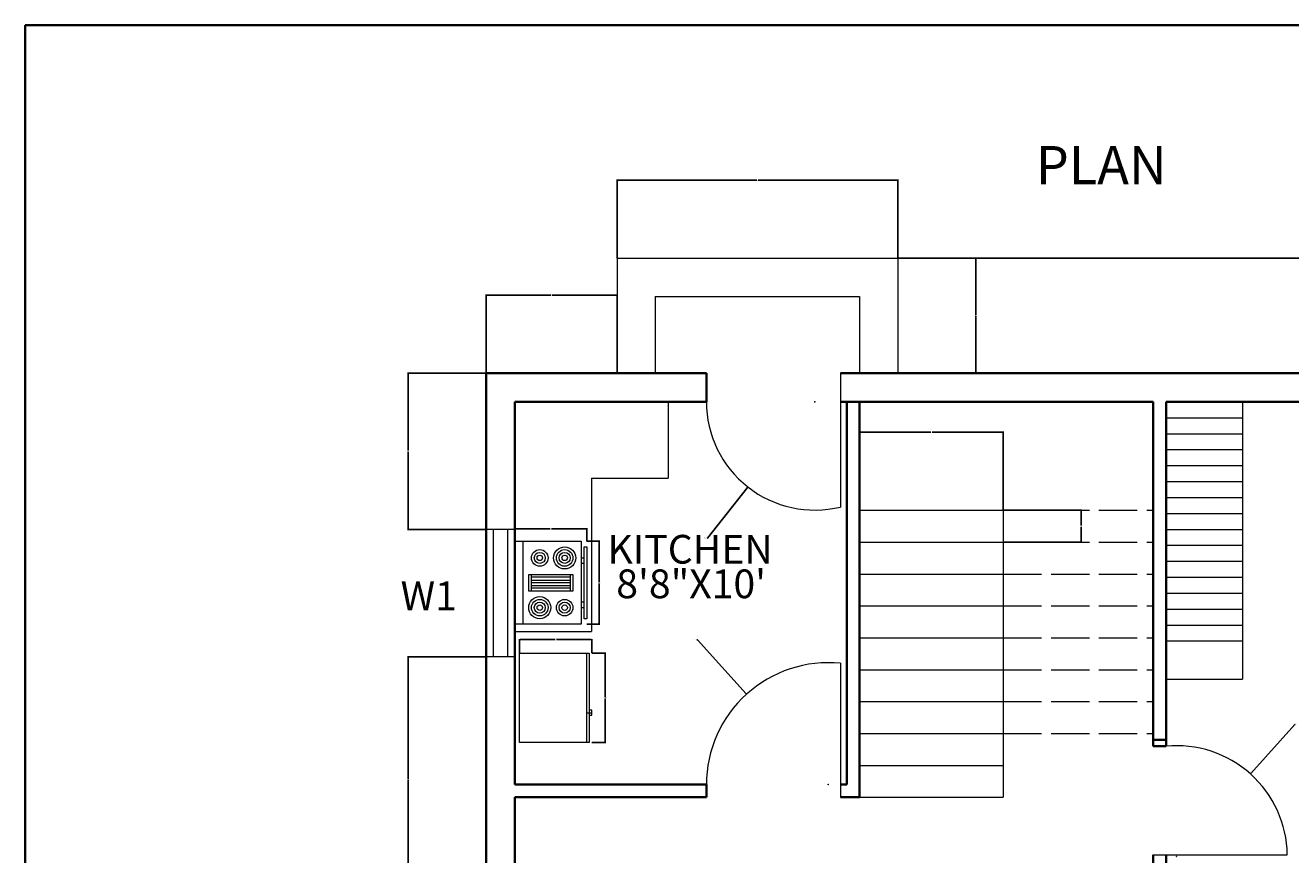
# Model space of a CAD drawing. Units: inches. Extents: x 2473 to 3664, y 1231 to 2079.
# Tile 5 of 8: x 2473 to 2870, y 1819 to 2079. Entities that reach past the tile are written whole.
import ezdxf

# ---------------------------------------------------------------- set-up
doc = ezdxf.new("R2010")
doc.units = ezdxf.units.IN
doc.linetypes.add('ACAD_ISO02W100', pattern=[15, 12, -3])
doc.layers.get('Defpoints').update_dxf_attribs({"linetype": 'ACAD_ISO02W100'})
for name, color, linetype, lineweight in [('A-ANNO-DIMS', 2, 'Continuous', 18), ('A-ANNO-IDEN', 7, 'Continuous', 18), ('A-ANNO-TEXT', 4, 'Continuous', 25), ('A-ANNO-TTLB', 7, 'Continuous', 35), ('A-AREA-IDEN', 7, 'Continuous', 18), ('A-DOOR', 4, 'Continuous', 18), ('A-EQPM', 8, 'Continuous', 18), ('A-FLOR-CASE', 9, 'Continuous', 18), ('A-FLOR-STRS', 7, 'Continuous', 18), ('A-FLOR-STRS-OVHD', 7, 'ACAD_ISO02W100', 13), ('A-GLAZ', 3, 'Continuous', 18), ('A-WALL', 7, 'Continuous', 35)]:
    doc.layers.add(name, color=color, linetype=linetype, lineweight=lineweight)
doc.styles.get("Standard").update_dxf_attribs({"font": 'arial.ttf'})
doc.dimstyles.get("Standard").update_dxf_attribs({"dimtxt": 0.18, "dimasz": 0.18, "dimexe": 0.18, "dimexo": 0.0625, "dimgap": 0.09, "dimtad": 0, "dimtih": 1, "dimtoh": 1, "dimdec": 4, "dimzin": 0, "dimdsep": 46, "dimtxsty": 'Standard', "dimcen": 0.09, "dimadec": 0, "dimazin": 0, "dimtfac": 1, "dimtdec": 4, "dimtofl": 0, "dimtmove": 0, "dimatfit": 3, "dimfxl": 1, "dimtolj": 1, "dimtzin": 0, "dimarcsym": 0})

# ---------------------------------------------------------------- blocks, each defined once
blk = doc.blocks.new('Range-Oven - 30 in top')
for p, q in [((0, -3), (30, -3)), ((12, -6), (18, -6)), ((13, -20), (13, -6)), ((14, -6), (14, -20)), ((15, -20), (15, -6)), ((16, -6), (16, -20)), ((17, -20), (17, -6)), ((18, -20), (12, -20)), ((6, -24), (6, -25)), ((8, -25), (8, -24)), ((22, -25), (22, -24)), ((24, -24), (24, -25))]:
    blk.add_line(p, q)
for points in [[(0, -24), (0, 0), (30, 0), (30, -24)], [(12, -21), (12, -5), (18, -5), (18, -21)], [(2, -26), (2, -25), (28, -25), (28, -26)]]:
    blk.add_lwpolyline(points, close=True)
for centre, radius in [((6, -9), 4), ((6, -9), 3), ((6, -9), 2), ((6, -9), 1), ((24, -9), 3), ((24, -9), 2), ((24, -9), 1), ((6, -18), 3), ((6, -18), 2), ((6, -18), 1), ((24, -18), 4), ((24, -18), 3), ((24, -18), 2), ((24, -18), 1)]:
    blk.add_circle(centre, radius)
blk = doc.blocks.new('Refrigerator-2 door - 36 in top')
for p, q in [((0, -26.999999), (36, -26.999999)), ((11, -27.999999), (11, -28.999999)), ((11, -28.999999), (13, -28.999999)), ((12, -26.999999), (12, -28.999999)), ((13, -28.999999), (13, -27.999999))]:
    blk.add_line(p, q)
blk.add_lwpolyline([(0, -27.999999), (0, 0), (36, 0), (36, -27.999999)], close=True)
blk = doc.blocks.new('GLAZ-PLAN-40')
for p, q in [((0, 40), (9, 40)), ((2.25, 40), (2.25, 0)), ((6.75, 40), (6.75, 0)), ((0, 0), (9, 0))]:
    blk.add_line(p, q)
blk = doc.blocks.new('*D37')
at = {"layer": 'A-ANNO-DIMS', "color": 0, "lineweight": -2, "transparency": 16777216}
for p, q in [((2649.25, 1917.31), (2653.27, 1917.31)), ((2653.09, 1917.13), (2653.09, 1904.49)), ((2653.09, 1891.49), (2653.09, 1904.13)), ((2649.25, 1891.31), (2653.27, 1891.31))]:
    blk.add_line(p, q, dxfattribs=at)
at = {"layer": 'A-ANNO-DIMS', "color": 0, "transparency": 16777216}
for points in [[(2653.06, 1917.13), (2653.12, 1917.13), (2653.09, 1917.31)], [(2653.06, 1891.49), (2653.12, 1891.49), (2653.09, 1891.31)]]:
    blk.add_solid(points, dxfattribs=at)
at = {"layer": 'Defpoints', "color": 0, "transparency": 16777216}
for p in [(2649.19, 1917.31), (2653.09, 1917.31), (2649.19, 1891.31)]:
    blk.add_point(p, dxfattribs=at)
at = {"layer": 'A-ANNO-DIMS', "color": 0, "transparency": 16777216, "insert": (2653.09, 1904.31), "char_height": 0.18, "attachment_point": 5}
blk.add_mtext('\\A1;RANGE 26', dxfattribs=at)
blk = doc.blocks.new('*D38')
at = {"layer": 'A-ANNO-DIMS', "color": 0, "lineweight": -2, "transparency": 16777216}
for p, q in [((2626.66, 1917.37), (2626.66, 1921.39)), ((2626.84, 1921.21), (2637.7, 1921.21)), ((2649.01, 1921.21), (2638.15, 1921.21)), ((2649.19, 1917.37), (2649.19, 1921.39))]:
    blk.add_line(p, q, dxfattribs=at)
at = {"layer": 'A-ANNO-DIMS', "color": 0, "transparency": 16777216}
for points in [[(2626.84, 1921.24), (2626.84, 1921.18), (2626.66, 1921.21)], [(2649.01, 1921.24), (2649.01, 1921.18), (2649.19, 1921.21)]]:
    blk.add_solid(points, dxfattribs=at)
at = {"layer": 'Defpoints', "color": 0, "transparency": 16777216}
for p in [(2626.66, 1921.21), (2626.66, 1917.31), (2649.19, 1917.31)]:
    blk.add_point(p, dxfattribs=at)
at = {"layer": 'A-ANNO-DIMS', "color": 0, "transparency": 16777216, "insert": (2637.93, 1921.21), "char_height": 0.18, "attachment_point": 5}
blk.add_mtext('\\A1;23', dxfattribs=at)
blk = doc.blocks.new('*D45')
at = {"layer": 'A-ANNO-DIMS', "color": 0, "lineweight": -2, "transparency": 16777216}
for p, q in [((2650.81, 1882.28), (2655.14, 1882.28)), ((2654.96, 1882.1), (2654.96, 1868.44)), ((2654.96, 1854.41), (2654.96, 1868.07)), ((2650.81, 1854.23), (2655.14, 1854.23))]:
    blk.add_line(p, q, dxfattribs=at)
at = {"layer": 'A-ANNO-DIMS', "color": 0, "transparency": 16777216}
for points in [[(2654.93, 1882.1), (2654.99, 1882.1), (2654.96, 1882.28)], [(2654.93, 1854.41), (2654.99, 1854.41), (2654.96, 1854.23)]]:
    blk.add_solid(points, dxfattribs=at)
at = {"layer": 'Defpoints', "color": 0, "transparency": 16777216}
for p in [(2650.75, 1882.28), (2654.96, 1882.28), (2650.75, 1854.23)]:
    blk.add_point(p, dxfattribs=at)
at = {"layer": 'A-ANNO-DIMS', "color": 0, "transparency": 16777216, "insert": (2654.96, 1868.26), "char_height": 0.18, "attachment_point": 5}
blk.add_mtext('\\A1;FRIDGE 28', dxfattribs=at)
blk = doc.blocks.new('*D46')
at = {"layer": 'A-ANNO-DIMS', "color": 0, "lineweight": -2, "transparency": 16777216}
for p, q in [((2628.15, 1882.35), (2628.15, 1886.67)), ((2628.33, 1886.49), (2639.23, 1886.49)), ((2650.57, 1886.49), (2639.67, 1886.49)), ((2650.75, 1882.35), (2650.75, 1886.67))]:
    blk.add_line(p, q, dxfattribs=at)
at = {"layer": 'A-ANNO-DIMS', "color": 0, "transparency": 16777216}
for points in [[(2628.33, 1886.52), (2628.33, 1886.46), (2628.15, 1886.49)], [(2650.57, 1886.52), (2650.57, 1886.46), (2650.75, 1886.49)]]:
    blk.add_solid(points, dxfattribs=at)
at = {"layer": 'Defpoints', "color": 0, "transparency": 16777216}
for p in [(2628.15, 1886.49), (2628.15, 1882.28), (2650.75, 1882.28)]:
    blk.add_point(p, dxfattribs=at)
at = {"layer": 'A-ANNO-DIMS', "color": 0, "transparency": 16777216, "insert": (2639.45, 1886.49), "char_height": 0.18, "attachment_point": 5}
blk.add_mtext('\\A1;23', dxfattribs=at)
blk = doc.blocks.new('*D50')
at = {"layer": 'A-ANNO-DIMS', "color": 0, "lineweight": -2, "transparency": 16777216}
for p, q in [((2746.72, 2006.06), (3020.29, 2006.06)), ((3020.11, 2005.88), (3020.11, 1797.24)), ((3020.11, 1588.24), (3020.11, 1796.87)), ((2844.72, 1588.06), (3020.29, 1588.06))]:
    blk.add_line(p, q, dxfattribs=at)
at = {"layer": 'A-ANNO-DIMS', "color": 0, "transparency": 16777216}
for points in [[(3020.08, 2005.88), (3020.14, 2005.88), (3020.11, 2006.06)], [(3020.08, 1588.24), (3020.14, 1588.24), (3020.11, 1588.06)]]:
    blk.add_solid(points, dxfattribs=at)
at = {"layer": 'Defpoints', "color": 0, "transparency": 16777216}
for p in [(2746.66, 2006.06), (3020.11, 2006.06), (2844.66, 1588.06)]:
    blk.add_point(p, dxfattribs=at)
at = {"layer": 'A-ANNO-DIMS', "color": 0, "transparency": 16777216, "insert": (3020.11, 1797.06), "char_height": 0.18, "attachment_point": 5}
blk.add_mtext('\\A1;418', dxfattribs=at)
blk = doc.blocks.new('*D51')
at = {"layer": 'A-ANNO-DIMS', "color": 0, "lineweight": -2, "transparency": 16777216}
for p, q in [((2746.72, 2006.06), (2771.29, 2006.06)), ((2771.11, 2005.88), (2771.11, 1988.24)), ((2771.11, 1970.24), (2771.11, 1987.87)), ((2746.72, 1970.06), (2771.29, 1970.06))]:
    blk.add_line(p, q, dxfattribs=at)
at = {"layer": 'A-ANNO-DIMS', "color": 0, "transparency": 16777216}
for points in [[(2771.08, 2005.88), (2771.14, 2005.88), (2771.11, 2006.06)], [(2771.08, 1970.24), (2771.14, 1970.24), (2771.11, 1970.06)]]:
    blk.add_solid(points, dxfattribs=at)
at = {"layer": 'Defpoints', "color": 0, "transparency": 16777216}
for p in [(2746.66, 2006.06), (2746.66, 1970.06), (2771.11, 1970.06)]:
    blk.add_point(p, dxfattribs=at)
at = {"layer": 'A-ANNO-DIMS', "color": 0, "transparency": 16777216, "insert": (2771.11, 1988.06), "char_height": 0.18, "attachment_point": 5}
blk.add_mtext('\\A1;36', dxfattribs=at)
blk = doc.blocks.new('*D53')
at = {"layer": 'A-ANNO-DIMS', "color": 0, "lineweight": -2, "transparency": 16777216}
for p, q in [((2658.66, 2006.12), (2658.66, 2030.69)), ((2658.84, 2030.51), (2702.44, 2030.51)), ((2746.48, 2030.51), (2702.88, 2030.51)), ((2746.66, 2006.12), (2746.66, 2030.69))]:
    blk.add_line(p, q, dxfattribs=at)
at = {"layer": 'A-ANNO-DIMS', "color": 0, "transparency": 16777216}
for points in [[(2658.84, 2030.54), (2658.84, 2030.48), (2658.66, 2030.51)], [(2746.48, 2030.54), (2746.48, 2030.48), (2746.66, 2030.51)]]:
    blk.add_solid(points, dxfattribs=at)
at = {"layer": 'Defpoints', "color": 0, "transparency": 16777216}
for p in [(2746.66, 2030.51), (2658.66, 2006.06), (2746.66, 2006.06)]:
    blk.add_point(p, dxfattribs=at)
at = {"layer": 'A-ANNO-DIMS', "color": 0, "transparency": 16777216, "insert": (2702.66, 2030.51), "char_height": 0.18, "attachment_point": 5}
blk.add_mtext('\\A1;88', dxfattribs=at)
blk = doc.blocks.new('*D54')
at = {"layer": 'A-ANNO-DIMS', "color": 0, "lineweight": -2, "transparency": 16777216}
for p, q in [((2617.66, 1970.12), (2617.66, 1994.69)), ((2617.84, 1994.51), (2637.96, 1994.51)), ((2658.48, 1994.51), (2638.37, 1994.51)), ((2658.66, 1970.12), (2658.66, 1994.69))]:
    blk.add_line(p, q, dxfattribs=at)
at = {"layer": 'A-ANNO-DIMS', "color": 0, "transparency": 16777216}
for points in [[(2617.84, 1994.54), (2617.84, 1994.48), (2617.66, 1994.51)], [(2658.48, 1994.54), (2658.48, 1994.48), (2658.66, 1994.51)]]:
    blk.add_solid(points, dxfattribs=at)
at = {"layer": 'Defpoints', "color": 0, "transparency": 16777216}
for p in [(2658.66, 1994.51), (2617.66, 1970.06), (2658.66, 1970.06)]:
    blk.add_point(p, dxfattribs=at)
at = {"layer": 'A-ANNO-DIMS', "color": 0, "transparency": 16777216, "insert": (2638.16, 1994.51), "char_height": 0.18, "attachment_point": 5}
blk.add_mtext('\\A1;41', dxfattribs=at)
blk = doc.blocks.new('*D59')
at = {"layer": 'A-ANNO-DIMS', "color": 0, "lineweight": -2, "transparency": 16777216}
for p, q in [((2617.597908, 1881.056109), (2593.030408, 1881.056109)), ((2593.210408, 1880.876109), (2593.210408, 1842.736109)), ((2593.210408, 1804.236109), (2593.210408, 1842.376109)), ((2617.597908, 1804.056109), (2593.030408, 1804.056109))]:
    blk.add_line(p, q, dxfattribs=at)
at = {"layer": 'A-ANNO-DIMS', "color": 0, "transparency": 16777216}
for points in [[(2593.180408, 1880.876109), (2593.240408, 1880.876109), (2593.210408, 1881.056109)], [(2593.180408, 1804.236109), (2593.240408, 1804.236109), (2593.210408, 1804.056109)]]:
    blk.add_solid(points, dxfattribs=at)
at = {"layer": 'Defpoints', "color": 0, "transparency": 16777216}
for p in [(2593.210408, 1881.056109), (2617.660408, 1881.056109), (2617.660408, 1804.056109)]:
    blk.add_point(p, dxfattribs=at)
at = {"layer": 'A-ANNO-DIMS', "color": 0, "transparency": 16777216, "insert": (2593.210408, 1842.556109), "char_height": 0.18, "attachment_point": 5}
blk.add_mtext('\\A1;77', dxfattribs=at)
blk = doc.blocks.new('*D60')
at = {"layer": 'A-ANNO-DIMS', "color": 0, "lineweight": -2, "transparency": 16777216}
for p, q in [((2617.6, 1970.06), (2593.03, 1970.06)), ((2593.21, 1969.88), (2593.21, 1945.74)), ((2593.21, 1921.24), (2593.21, 1945.37)), ((2617.6, 1921.06), (2593.03, 1921.06))]:
    blk.add_line(p, q, dxfattribs=at)
at = {"layer": 'A-ANNO-DIMS', "color": 0, "transparency": 16777216}
for points in [[(2593.18, 1969.88), (2593.24, 1969.88), (2593.21, 1970.06)], [(2593.18, 1921.24), (2593.24, 1921.24), (2593.21, 1921.06)]]:
    blk.add_solid(points, dxfattribs=at)
at = {"layer": 'Defpoints', "color": 0, "transparency": 16777216}
for p in [(2593.21, 1970.06), (2617.66, 1970.06), (2617.66, 1921.06)]:
    blk.add_point(p, dxfattribs=at)
at = {"layer": 'A-ANNO-DIMS', "color": 0, "transparency": 16777216, "insert": (2593.21, 1945.56), "char_height": 0.18, "attachment_point": 5}
blk.add_mtext('\\A1;49', dxfattribs=at)
blk = doc.blocks.new('*D63')
at = {"layer": 'A-ANNO-DIMS', "color": 0, "lineweight": -2, "transparency": 16777216}
for p, q in [((2734.66, 1927.12), (2734.66, 1951.69)), ((2734.84, 1951.51), (2756.94, 1951.51)), ((2779.48, 1951.51), (2757.38, 1951.51)), ((2779.66, 1927.12), (2779.66, 1951.69))]:
    blk.add_line(p, q, dxfattribs=at)
at = {"layer": 'A-ANNO-DIMS', "color": 0, "transparency": 16777216}
for points in [[(2734.84, 1951.54), (2734.84, 1951.48), (2734.66, 1951.51)], [(2779.48, 1951.54), (2779.48, 1951.48), (2779.66, 1951.51)]]:
    blk.add_solid(points, dxfattribs=at)
at = {"layer": 'Defpoints', "color": 0, "transparency": 16777216}
for p in [(2779.66, 1951.51), (2734.66, 1927.06), (2779.66, 1927.06)]:
    blk.add_point(p, dxfattribs=at)
at = {"layer": 'A-ANNO-DIMS', "color": 0, "transparency": 16777216, "insert": (2757.16, 1951.51), "char_height": 0.18, "attachment_point": 5}
blk.add_mtext('\\A1;45', dxfattribs=at)
blk = doc.blocks.new('*D64')
at = {"layer": 'A-ANNO-DIMS', "color": 0, "lineweight": -2, "transparency": 16777216}
for p, q in [((2779.72, 1927.06), (2804.29, 1927.06)), ((2804.11, 1926.88), (2804.11, 1922.24)), ((2804.11, 1917.24), (2804.11, 1921.87)), ((2779.72, 1917.06), (2804.29, 1917.06))]:
    blk.add_line(p, q, dxfattribs=at)
at = {"layer": 'A-ANNO-DIMS', "color": 0, "transparency": 16777216}
for points in [[(2804.08, 1926.88), (2804.14, 1926.88), (2804.11, 1927.06)], [(2804.08, 1917.24), (2804.14, 1917.24), (2804.11, 1917.06)]]:
    blk.add_solid(points, dxfattribs=at)
at = {"layer": 'Defpoints', "color": 0, "transparency": 16777216}
for p in [(2779.66, 1927.06), (2779.66, 1917.06), (2804.11, 1917.06)]:
    blk.add_point(p, dxfattribs=at)
at = {"layer": 'A-ANNO-DIMS', "color": 0, "transparency": 16777216, "insert": (2804.11, 1922.06), "char_height": 0.18, "attachment_point": 5}
blk.add_mtext('\\A1;10', dxfattribs=at)
blk = doc.blocks.new('*D107')
at = {"layer": 'A-ANNO-DIMS', "color": 0, "lineweight": -2, "transparency": 16777216}
for p, q in [((2683.67, 1886.37), (2683.85, 1886.37)), ((2683.85, 1886.37), (2699.11, 1869.51)), ((2724.76, 1841.06), (2724.94, 1841.06)), ((2724.85, 1840.97), (2724.85, 1841.15))]:
    blk.add_line(p, q, dxfattribs=at)
at = {"layer": 'A-ANNO-DIMS', "color": 0, "transparency": 16777216}
blk.add_solid([(2699.13, 1869.53), (2699.09, 1869.49), (2699.23, 1869.38)], dxfattribs=at)
at = {"layer": 'Defpoints', "color": 0, "transparency": 16777216}
for p in [(2699.23, 1869.38), (2724.85, 1841.06)]:
    blk.add_point(p, dxfattribs=at)
at = {"layer": 'A-ANNO-DIMS', "color": 0, "transparency": 16777216, "insert": (2683.19, 1886.37), "char_height": 0.18, "attachment_point": 5}
blk.add_mtext('\\A1;R38.19', dxfattribs=at)
blk = doc.blocks.new('*D108')
at = {"layer": 'A-ANNO-DIMS', "color": 0, "lineweight": -2, "transparency": 16777216}
for p, q in [((2870.98, 1859.89), (2857.23, 1844.52)), ((2871.16, 1859.89), (2870.98, 1859.89)), ((2833.9, 1818.54), (2834.08, 1818.54)), ((2833.99, 1818.45), (2833.99, 1818.63))]:
    blk.add_line(p, q, dxfattribs=at)
at = {"layer": 'A-ANNO-DIMS', "color": 0, "transparency": 16777216}
blk.add_solid([(2857.21, 1844.54), (2857.25, 1844.5), (2857.11, 1844.38)], dxfattribs=at)
at = {"layer": 'Defpoints', "color": 0, "transparency": 16777216}
for p in [(2857.11, 1844.38), (2833.99, 1818.54)]:
    blk.add_point(p, dxfattribs=at)
at = {"layer": 'A-ANNO-DIMS', "color": 0, "transparency": 16777216, "insert": (2871.64, 1859.89), "char_height": 0.18, "attachment_point": 5}
blk.add_mtext('\\A1;R34.68', dxfattribs=at)
blk = doc.blocks.new('*D109')
at = {"layer": 'A-ANNO-DIMS', "color": 0, "lineweight": -2, "transparency": 16777216}
for p, q in [((2720.53, 1961.06), (2720.71, 1961.06)), ((2720.62, 1960.97), (2720.62, 1961.15)), ((2687.05, 1918.32), (2699.53, 1934.21)), ((2686.87, 1918.32), (2687.05, 1918.32))]:
    blk.add_line(p, q, dxfattribs=at)
at = {"layer": 'A-ANNO-DIMS', "color": 0, "transparency": 16777216}
blk.add_solid([(2699.51, 1934.23), (2699.55, 1934.19), (2699.64, 1934.35)], dxfattribs=at)
at = {"layer": 'Defpoints', "color": 0, "transparency": 16777216}
for p in [(2720.62, 1961.06), (2699.64, 1934.35)]:
    blk.add_point(p, dxfattribs=at)
at = {"layer": 'A-ANNO-DIMS', "color": 0, "transparency": 16777216, "insert": (2686.32, 1918.32), "char_height": 0.18, "attachment_point": 5}
blk.add_mtext('\\A1;R33.964', dxfattribs=at)

msp = doc.modelspace()

# ---------------------------------------------------------------- linework, layer by layer
at = {"layer": 'A-ANNO-TTLB'}
msp.add_lwpolyline([(2473.2801, 2079.0861), (3663.7983, 2079.0861), (3663.7983, 1231.3065), (2473.2801, 1231.3065)], close=True, dxfattribs=at)
at = {"layer": 'A-DOOR'}
for p, q in [((2728.6604, 1970.0561), (2728.6604, 1928.0561)), ((2728.6604, 1879.0561), (2728.6604, 1837.0561)), ((2826.6604, 1819.0561), (2868.6604, 1819.0561))]:
    msp.add_line(p, q, dxfattribs=at)
for centre, radius, start, end in [((2720.6247, 1961.0561), 33.9643, 180, 283.685547), ((2724.8509, 1841.0561), 38.1905, 84.27519, 180), ((2833.9877, 1818.5395), 34.6766, 0.853554, 95.506107)]:
    msp.add_arc(centre, radius, start, end, dxfattribs=at)
at = {"layer": 'A-FLOR-CASE'}
for p, q in [((2674.6604, 1961.0561), (2674.6604, 1937.0561)), ((2854.6604, 1961.0561), (2854.6604, 1874.0561)), ((2830.6604, 1956.0561), (2854.6604, 1956.0561)), ((2830.6604, 1951.0561), (2854.6604, 1951.0561)), ((2830.6604, 1946.0561), (2854.6604, 1946.0561)), ((2830.6604, 1941.0561), (2854.6604, 1941.0561)), ((2650.6604, 1937.0561), (2650.6604, 1889.0561)), ((2650.6604, 1937.0561), (2674.6604, 1937.0561)), ((2830.6604, 1936.0561), (2854.6604, 1936.0561)), ((2830.6604, 1931.0561), (2854.6604, 1931.0561)), ((2830.6604, 1926.0561), (2854.6604, 1926.0561)), ((2830.6604, 1921.0561), (2854.6604, 1921.0561)), ((2830.6604, 1916.0561), (2854.6604, 1916.0561)), ((2830.6604, 1911.0561), (2854.6604, 1911.0561)), ((2830.6604, 1906.0561), (2854.6604, 1906.0561)), ((2830.6604, 1901.0561), (2854.6604, 1901.0561)), ((2830.6604, 1896.0561), (2854.6604, 1896.0561)), ((2830.6604, 1891.0561), (2854.6604, 1891.0561)), ((2626.6604, 1889.0561), (2650.6604, 1889.0561)), ((2830.6604, 1886.0561), (2854.6604, 1886.0561)), ((2830.6604, 1874.0561), (2854.6604, 1874.0561))]:
    msp.add_line(p, q, dxfattribs=at)
at = {"layer": 'A-FLOR-STRS'}
for p, q in [((2658.6604, 2006.0561), (2746.6604, 2006.0561)), ((2658.6604, 2006.0561), (2658.6604, 1970.0561)), ((2746.6604, 2006.0561), (2746.6604, 1970.0561)), ((2670.6604, 1994.0561), (2670.6604, 1970.0561)), ((2670.6604, 1994.0561), (2734.6604, 1994.0561)), ((2734.6604, 1994.0561), (2734.6604, 1970.0561)), ((2734.6604, 1927.0561), (2779.6604, 1927.0561)), ((2779.6604, 1927.0561), (2779.6604, 1837.0561)), ((2734.6604, 1917.0561), (2779.6604, 1917.0561)), ((2734.6604, 1907.0561), (2779.6604, 1907.0561)), ((2734.6604, 1897.0561), (2779.6604, 1897.0561)), ((2734.6604, 1887.0561), (2779.6604, 1887.0561)), ((2734.6604, 1877.0561), (2779.6604, 1877.0561)), ((2734.6604, 1867.0561), (2779.6604, 1867.0561)), ((2734.6604, 1857.0561), (2779.6604, 1857.0561)), ((2734.6604, 1847.0561), (2779.6604, 1847.0561)), ((2734.6604, 1837.0561), (2779.6604, 1837.0561))]:
    msp.add_line(p, q, dxfattribs=at)
at = {"layer": 'A-FLOR-STRS-OVHD'}
for p, q in [((2779.6604, 1927.0561), (2826.6604, 1927.0561)), ((2779.6604, 1917.0561), (2826.6604, 1917.0561)), ((2779.6604, 1907.0561), (2826.6604, 1907.0561)), ((2779.6604, 1897.0561), (2826.6604, 1897.0561)), ((2779.6604, 1887.0561), (2826.6604, 1887.0561)), ((2779.6604, 1877.0561), (2826.6604, 1877.0561)), ((2779.6604, 1867.0561), (2826.6604, 1867.0561)), ((2779.6604, 1857.0561), (2826.6604, 1857.0561))]:
    msp.add_line(p, q, dxfattribs=at)
at = {"layer": 'A-WALL'}
for p, q in [((2617.6604, 1970.0561), (2686.6604, 1970.0561)), ((2617.6604, 1970.0561), (2617.6604, 1588.0561)), ((2686.6604, 1970.0561), (2686.6604, 1961.0561)), ((2728.6604, 1970.0561), (2995.6604, 1970.0561)), ((2626.6604, 1961.0561), (2686.6604, 1961.0561)), ((2626.6604, 1961.0561), (2626.6604, 1841.0561)), ((2728.6604, 1961.0561), (2826.6604, 1961.0561)), ((2730.6604, 1961.0561), (2730.6604, 1841.0561)), ((2734.6604, 1961.0561), (2734.6604, 1837.0561)), ((2826.6604, 1961.0561), (2826.6604, 1853.0561)), ((2826.6604, 1961.0561), (2826.6604, 1855.0561)), ((2830.6604, 1961.0561), (2830.6604, 1853.0561)), ((2830.6604, 1961.0561), (2995.6604, 1961.0561)), ((2830.6604, 1956.0561), (2830.6604, 1855.0561)), ((2830.6604, 1956.0561), (2830.6604, 1855.0561)), ((2826.6604, 1855.0561), (2830.6604, 1855.0561)), ((2826.6604, 1853.0561), (2830.6604, 1853.0561)), ((2626.6604, 1841.0561), (2686.6604, 1841.0561)), ((2686.6604, 1841.0561), (2686.6604, 1837.0561)), ((2728.6604, 1841.0561), (2730.6604, 1841.0561)), ((2626.6604, 1837.0561), (2686.6604, 1837.0561)), ((2626.6604, 1837.0561), (2626.6604, 1721.0561)), ((2728.6604, 1837.0561), (2734.6604, 1837.0561)), ((2826.6604, 1819.0561), (2826.6604, 1813.0561)), ((2826.6604, 1819.0561), (2826.6604, 1813.0561)), ((2830.6604, 1819.0561), (2830.6604, 1813.0561)), ((2830.6604, 1819.0561), (2830.6604, 1813.0561)), ((2830.6604, 1819.0561), (2830.6604, 1813.0561))]:
    msp.add_line(p, q, dxfattribs=at)

# ---------------------------------------------------------------- block references
at = {"layer": 'A-EQPM', "rotation": 90}
for name, p, xscale, yscale, zscale in [('Range-Oven - 30 in top', (2626.6589, 1891.3091), 0.8666231730426178, 0.8666231730426178, 0.8666231730426178), ('Refrigerator-2 door - 36 in top', (2628.1525, 1854.2304), 0.7792515062667271, 0.7792515062667271, 0.7792515062667271)]:
    msp.add_blockref(name, p, dxfattribs=dict(at, xscale=xscale, yscale=yscale, zscale=zscale))
at = {"layer": 'A-GLAZ', "rotation": 180}
msp.add_blockref('GLAZ-PLAN-40', (2626.6608, 1921.0562), dxfattribs=at)

# ---------------------------------------------------------------- texts
at = {"layer": 'A-ANNO-IDEN'}
msp.add_text('           W1', height=9, dxfattribs=at).set_placement((2560.6171, 1895.7183))
at = {"layer": 'A-ANNO-TEXT'}
msp.add_text('PLAN', height=12, dxfattribs=at).set_placement((2789.8466, 2029.238))
at = {"layer": 'A-AREA-IDEN'}
for s, p in [('KITCHEN', (2655.6694, 1910.3203)), (' 8\'8"X10\'', (2655.6694, 1899.4821))]:
    msp.add_text(s, height=9, dxfattribs=at).set_placement(p)

# ---------------------------------------------------------------- dimensions: what is measured, and where the dimension line sits
at = {"layer": 'A-ANNO-DIMS'}
for base, p1, p2, picture, middle in [((2746.6604, 2030.5061), (2658.6604, 2006.0561), (2746.6604, 2006.0561), '*D53', (2702.6604, 2030.5061)), ((2658.6604, 1994.5061), (2617.6604, 1970.0561), (2658.6604, 1970.0561), '*D54', (2638.1604, 1994.5061)), ((2779.6604, 1951.5061), (2734.6604, 1927.0561), (2779.6604, 1927.0561), '*D63', (2757.1604, 1951.5061))]:
    dim = msp.add_linear_dim(base=base, p1=p1, p2=p2, dimstyle='Standard', override={"dimdec": 0, "dimlfac": 1, "dimrnd": 0, "dimzin": 0, "dimdsep": 46, "dimlunit": 2}, dxfattribs=at)
    dim.commit()
    dim.dimension.update_dxf_attribs({"geometry": picture, "text_midpoint": middle})
for base, p1, p2, angle, picture, middle in [((3020.1104, 2006.0561), (2844.6604, 1588.0561), (2746.6604, 2006.0561), 90, '*D50', (3020.1104, 1797.0561)), ((2771.1104, 1970.0561), (2746.6604, 2006.0561), (2746.6604, 1970.0561), 270, '*D51', (2771.1104, 1988.0561)), ((2593.2104, 1970.0561), (2617.6604, 1921.0561), (2617.6604, 1970.0561), 90, '*D60', (2593.2104, 1945.5561)), ((2804.1104, 1917.0561), (2779.6604, 1927.0561), (2779.6604, 1917.0561), 270, '*D64', (2804.1104, 1922.0561)), ((2626.6589, 1921.2076), (2649.1911, 1917.3078), (2626.6589, 1917.3078), 180, '*D38', (2637.925, 1921.2076)), ((2628.1525, 1886.4914), (2650.7508, 1882.2835), (2628.1525, 1882.2835), 180, '*D46', (2639.4516, 1886.4914)), ((2593.2104, 1881.0561), (2617.6604, 1804.0561), (2617.6604, 1881.0561), 90, '*D59', (2593.2104, 1842.5561))]:
    dim = msp.add_linear_dim(base=base, p1=p1, p2=p2, angle=angle, dimstyle='Standard', override={"dimdec": 0, "dimlfac": 1, "dimrnd": 0, "dimzin": 0, "dimdsep": 46, "dimlunit": 2}, dxfattribs=at)
    dim.commit()
    dim.dimension.update_dxf_attribs({"geometry": picture, "text_midpoint": middle})
for center, mpoint, override, picture, middle in [((2720.6247, 1961.0561), (2699.6411, 1934.3491), {"dimdec": 3, "dimlfac": 1, "dimrnd": 0, "dimzin": 0, "dimdsep": 46, "dimlunit": 2}, '*D109', (2686.3216, 1918.325)), ((2724.8509, 1841.0561), (2699.2283, 1869.3757), {"dimdec": 2, "dimlfac": 1, "dimrnd": 0, "dimzin": 0, "dimdsep": 46, "dimlunit": 2}, '*D107', (2683.1948, 1886.3674)), ((2833.9877, 1818.5395), (2857.1099, 1844.3819), {"dimdec": 2, "dimlfac": 1, "dimrnd": 0, "dimzin": 0, "dimdsep": 46, "dimlunit": 2}, '*D108', (2871.6433, 1859.8873))]:
    dim = msp.add_radius_dim(center=center, mpoint=mpoint, dimstyle='Standard', override=override, dxfattribs=at)
    dim.commit()
    dim.dimension.update_dxf_attribs({"geometry": picture, "text_midpoint": middle, "dimtype": 164})
for base, p1, p2, text, picture, middle in [((2653.0909, 1917.3078), (2649.1911, 1891.3091), (2649.1911, 1917.3078), 'RANGE <>', '*D37', (2653.0909, 1904.3084)), ((2654.9587, 1882.2835), (2650.7508, 1854.2304), (2650.7508, 1882.2835), 'FRIDGE <>', '*D45', (2654.9587, 1868.2569))]:
    dim = msp.add_linear_dim(base=base, p1=p1, p2=p2, angle=90, text=text, dimstyle='Standard', override={"dimdec": 0, "dimlfac": 1, "dimrnd": 0, "dimzin": 0, "dimdsep": 46, "dimlunit": 2}, dxfattribs=at)
    dim.commit()
    dim.dimension.update_dxf_attribs({"geometry": picture, "text_midpoint": middle})

doc.saveas('drawing.dxf')
